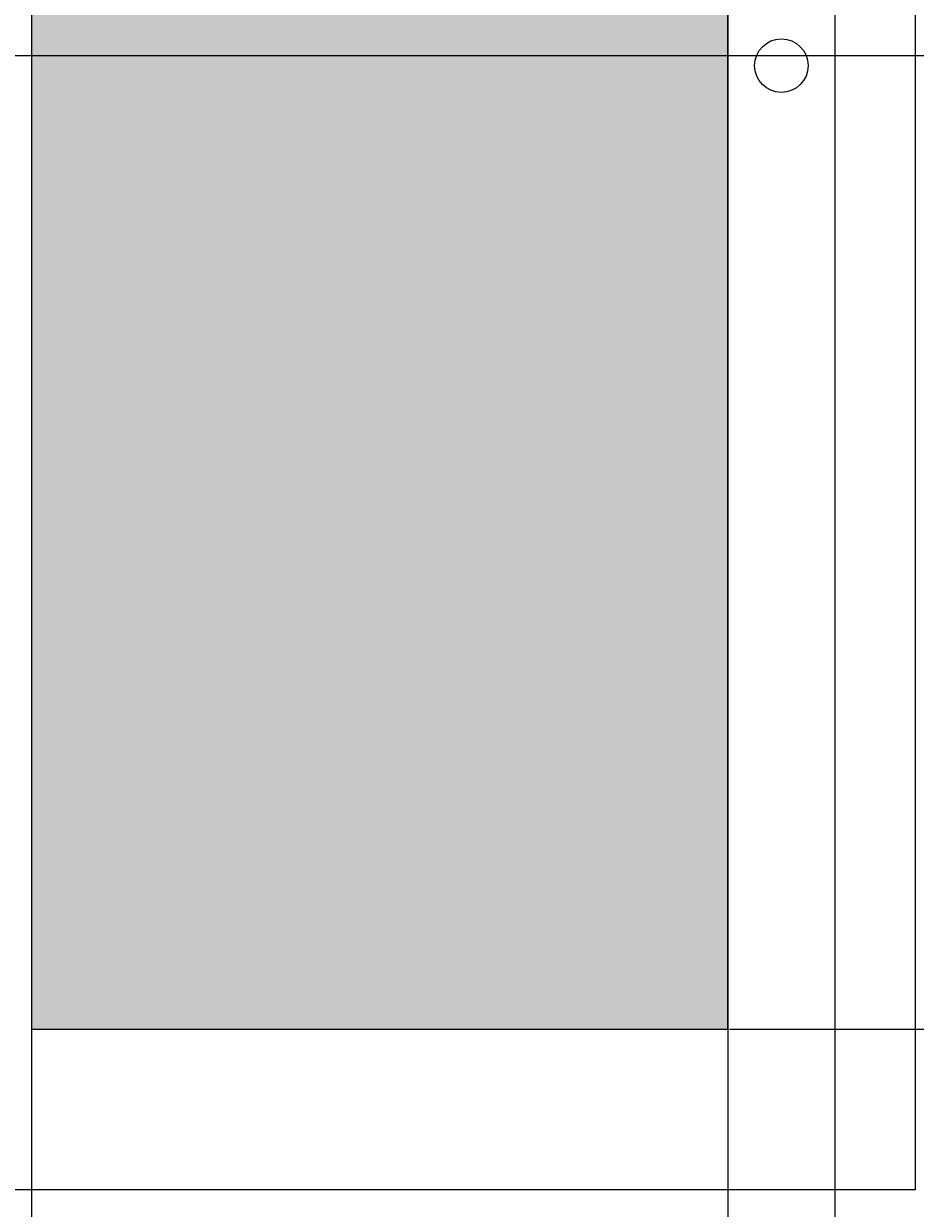
# Model space of a CAD drawing. Units: inches. Extents: x 37 to 824, y -700 to 234.
# Tile 13 of 77: x 315 to 348, y -581 to -536. Entities that reach past the tile are written whole.
import ezdxf

# ---------------------------------------------------------------- set-up
doc = ezdxf.new("R2010")
doc.units = ezdxf.units.IN
doc.header["$MEASUREMENT"] = 0
for name, color, linetype, lineweight in [('A-ANNO-DIMS', 2, 'Continuous', 18), ('A-DOOR', 4, 'Continuous', 25), ('A-ELEV-PATT', 8, 'Continuous', 13)]:
    doc.layers.add(name, color=color, linetype=linetype, lineweight=lineweight)
doc.styles.get("Standard").update_dxf_attribs({"font": 'arial.ttf'})
doc.dimstyles.get("Standard").update_dxf_attribs({"dimtxt": 0.18, "dimasz": 0.18, "dimexe": 0.18, "dimexo": 0.0625, "dimgap": 0.09, "dimtad": 0, "dimtih": 1, "dimtoh": 1, "dimdec": 1, "dimzin": 0, "dimdsep": 46, "dimlunit": 4, "dimtxsty": 'Standard', "dimcen": 0.09, "dimadec": 0, "dimazin": 0, "dimtfac": 1, "dimtdec": 1, "dimtofl": 0, "dimtmove": 0, "dimatfit": 3, "dimfxl": 1, "dimtolj": 1, "dimtzin": 0, "dimarcsym": 0})

# ---------------------------------------------------------------- blocks, each defined once
blk = doc.blocks.new('*U9')
blk.add_lwpolyline([(3.124, 0.013), (0.124, 0.013), (0.124, 84.013), (40.124, 84.013), (40.124, 0.013), (37.124, 0.013)])
for points in [[(37.124, 80.99), (37.124, 0.013), (3.124, 0.013), (3.124, 80.99)], [(33.124, 6.013), (33.124, 74.99), (7.124, 74.99), (7.124, 6.013)]]:
    blk.add_lwpolyline(points, close=True)
blk.add_circle((35.124, 42.013), 1)
blk = doc.blocks.new('*D28')
at = {"layer": 'A-ANNO-DIMS', "color": 0, "lineweight": -2, "ltscale": 0.5, "transparency": 16777216}
for p, q in [((255.14, -537.627), (449.868, -537.627)), ((449.688, -543.627), (449.688, -558.537)), ((449.688, -579.627), (449.688, -564.717)), ((294.64, -585.627), (449.868, -585.627))]:
    blk.add_line(p, q, dxfattribs=at)
at = {"layer": 'A-ANNO-DIMS', "color": 0, "ltscale": 0.5, "transparency": 16777216}
for points in [[(448.688, -543.627), (450.688, -543.627), (449.688, -537.627)], [(448.688, -579.627), (450.688, -579.627), (449.688, -585.627)]]:
    blk.add_solid(points, dxfattribs=at)
at = {"layer": 'Defpoints', "color": 0, "ltscale": 0.5, "transparency": 16777216}
for p in [(255.077, -537.627), (294.577, -585.627), (449.688, -585.627)]:
    blk.add_point(p, dxfattribs=at)
at = {"layer": 'A-ANNO-DIMS', "color": 0, "ltscale": 0.5, "transparency": 16777216, "insert": (449.688, -561.627), "char_height": 6, "attachment_point": 5}
blk.add_mtext("\\A1;4'", dxfattribs=at)
blk = doc.blocks.new('*D31')
at = {"layer": 'A-ANNO-DIMS', "color": 0, "lineweight": -2, "ltscale": 0.5, "transparency": 16777216}
for p, q in [((255.14, -489.627), (449.772, -489.627)), ((449.592, -495.627), (449.592, -510.537)), ((449.592, -531.627), (449.592, -516.717)), ((255.14, -537.627), (449.772, -537.627))]:
    blk.add_line(p, q, dxfattribs=at)
at = {"layer": 'A-ANNO-DIMS', "color": 0, "ltscale": 0.5, "transparency": 16777216}
for points in [[(448.592, -495.627), (450.592, -495.627), (449.592, -489.627)], [(448.592, -531.627), (450.592, -531.627), (449.592, -537.627)]]:
    blk.add_solid(points, dxfattribs=at)
at = {"layer": 'Defpoints', "color": 0, "ltscale": 0.5, "transparency": 16777216}
for p in [(255.077, -489.627), (449.592, -489.627), (255.077, -537.627)]:
    blk.add_point(p, dxfattribs=at)
at = {"layer": 'A-ANNO-DIMS', "color": 0, "ltscale": 0.5, "transparency": 16777216, "insert": (449.592, -513.627), "char_height": 6, "attachment_point": 5}
blk.add_mtext("\\A1;4'", dxfattribs=at)
blk = doc.blocks.new('*D102')
at = {"layer": 'A-ANNO-DIMS', "color": 0, "lineweight": -2, "ltscale": 0.5, "transparency": 16777216}
for p, q in [((311.196, -499.092), (311.196, -699.594)), ((345.196, -499.092), (345.196, -699.594)), ((311.376, -699.414), (327.795, -699.414)), ((345.016, -699.414), (328.596, -699.414))]:
    blk.add_line(p, q, dxfattribs=at)
at = {"layer": 'A-ANNO-DIMS', "color": 0, "ltscale": 0.5, "transparency": 16777216}
for points in [[(311.376, -699.384), (311.376, -699.444), (311.196, -699.414)], [(345.016, -699.384), (345.016, -699.444), (345.196, -699.414)]]:
    blk.add_solid(points, dxfattribs=at)
at = {"layer": 'Defpoints', "color": 0, "ltscale": 0.5, "transparency": 16777216}
for p in [(311.196, -499.03), (345.196, -499.03), (345.196, -699.414)]:
    blk.add_point(p, dxfattribs=at)
at = {"layer": 'A-ANNO-DIMS', "color": 0, "ltscale": 0.5, "transparency": 16777216, "insert": (328.196, -699.414), "char_height": 0.18, "attachment_point": 5}
blk.add_mtext('\\A1;2\'-10"', dxfattribs=at)
blk = doc.blocks.new('*D103')
at = {"layer": 'A-ANNO-DIMS', "color": 0, "lineweight": -2, "ltscale": 0.5, "transparency": 16777216}
for p, q in [((315.196, -505.092), (315.196, -699.594)), ((341.196, -505.092), (341.196, -699.594)), ((315.376, -699.414), (327.865, -699.414)), ((341.016, -699.414), (328.526, -699.414))]:
    blk.add_line(p, q, dxfattribs=at)
at = {"layer": 'A-ANNO-DIMS', "color": 0, "ltscale": 0.5, "transparency": 16777216}
for points in [[(315.376, -699.384), (315.376, -699.444), (315.196, -699.414)], [(341.016, -699.384), (341.016, -699.444), (341.196, -699.414)]]:
    blk.add_solid(points, dxfattribs=at)
at = {"layer": 'Defpoints', "color": 0, "ltscale": 0.5, "transparency": 16777216}
for p in [(315.196, -505.03), (341.196, -505.03), (341.196, -699.414)]:
    blk.add_point(p, dxfattribs=at)
at = {"layer": 'A-ANNO-DIMS', "color": 0, "ltscale": 0.5, "transparency": 16777216, "insert": (328.196, -699.414), "char_height": 0.18, "attachment_point": 5}
blk.add_mtext('\\A1;2\'-2"', dxfattribs=at)
blk = doc.blocks.new('*D104')
at = {"layer": 'A-ANNO-DIMS', "color": 0, "lineweight": -2, "ltscale": 0.5, "transparency": 16777216}
for p, q in [((341.258, -505.03), (556.923, -505.03)), ((556.743, -505.21), (556.743, -539.336)), ((556.743, -573.827), (556.743, -539.7)), ((341.258, -574.007), (556.923, -574.007))]:
    blk.add_line(p, q, dxfattribs=at)
at = {"layer": 'A-ANNO-DIMS', "color": 0, "ltscale": 0.5, "transparency": 16777216}
for points in [[(556.713, -505.21), (556.773, -505.21), (556.743, -505.03)], [(556.713, -573.827), (556.773, -573.827), (556.743, -574.007)]]:
    blk.add_solid(points, dxfattribs=at)
at = {"layer": 'Defpoints', "color": 0, "ltscale": 0.5, "transparency": 16777216}
for p in [(341.196, -505.03), (341.196, -574.007), (556.743, -574.007)]:
    blk.add_point(p, dxfattribs=at)
at = {"layer": 'A-ANNO-DIMS', "color": 0, "ltscale": 0.5, "transparency": 16777216, "insert": (556.743, -539.518), "char_height": 0.18, "attachment_point": 5}
blk.add_mtext('\\A1;5\'-9"', dxfattribs=at)

msp = doc.modelspace()

# ---------------------------------------------------------------- hatches: boundary and pattern name
at = {"layer": 'A-ELEV-PATT', "ltscale": 0.5}
h = msp.add_hatch(color=256, dxfattribs=at)
h.dxf.hatch_style = 1
h.paths.add_polyline_path([(161.077, -459.627), (161.077, -465.627), (428.077, -465.627), (428.077, -459.627)])
h.paths.add_polyline_path([(229.025, -498.214), (214.525, -498.214), (214.525, -529.214), (229.025, -529.214)])
h.paths.add_polyline_path([(245.525, -498.214), (230.025, -498.214), (230.025, -529.214), (245.525, -529.214)])
h.paths.add_polyline_path([(315.196, -574.007), (341.196, -574.007), (341.196, -505.03), (315.196, -505.03)])

# ---------------------------------------------------------------- block references
at = {"layer": 'A-DOOR'}
msp.add_blockref('*U9', (308.072, -580.019), dxfattribs=at)

# ---------------------------------------------------------------- dimensions: what is measured, and where the dimension line sits
at = {"layer": 'A-ANNO-DIMS', "ltscale": 0.5}
for base, p1, p2, override, picture, middle in [((449.592, -489.627), (255.077, -537.627), (255.077, -489.627), {"dimtxt": 6, "dimasz": 6, "dimclrd": 0, "dimclre": 0, "dimclrt": 0}, '*D31', (449.592, -513.627)), ((556.743, -574.007), (341.196, -505.03), (341.196, -574.007), {"dimdec": 1, "dimlfac": 1, "dimrnd": 0, "dimzin": 1, "dimdsep": 46, "dimlunit": 4, "dimfrac": 2}, '*D104', (556.743, -539.518)), ((449.688, -585.627), (255.077, -537.627), (294.577, -585.627), {"dimtxt": 6, "dimasz": 6, "dimclrd": 0, "dimclre": 0, "dimclrt": 0}, '*D28', (449.688, -561.627))]:
    dim = msp.add_linear_dim(base=base, p1=p1, p2=p2, angle=90, dimstyle='Standard', override=override, dxfattribs=at)
    dim.commit()
    dim.dimension.update_dxf_attribs({"geometry": picture, "text_midpoint": middle})
for base, p1, p2, picture in [((345.196, -699.414), (311.196, -499.03), (345.196, -499.03), '*D102'), ((341.196, -699.414), (315.196, -505.03), (341.196, -505.03), '*D103')]:
    dim = msp.add_linear_dim(base=base, p1=p1, p2=p2, dimstyle='Standard', override={"dimdec": 1, "dimlfac": 1, "dimrnd": 0, "dimzin": 1, "dimdsep": 46, "dimlunit": 4, "dimfrac": 2}, dxfattribs=at)
    dim.commit()
    dim.dimension.update_dxf_attribs({"geometry": picture, "text_midpoint": (328.196, -699.414)})

doc.saveas('drawing.dxf')
